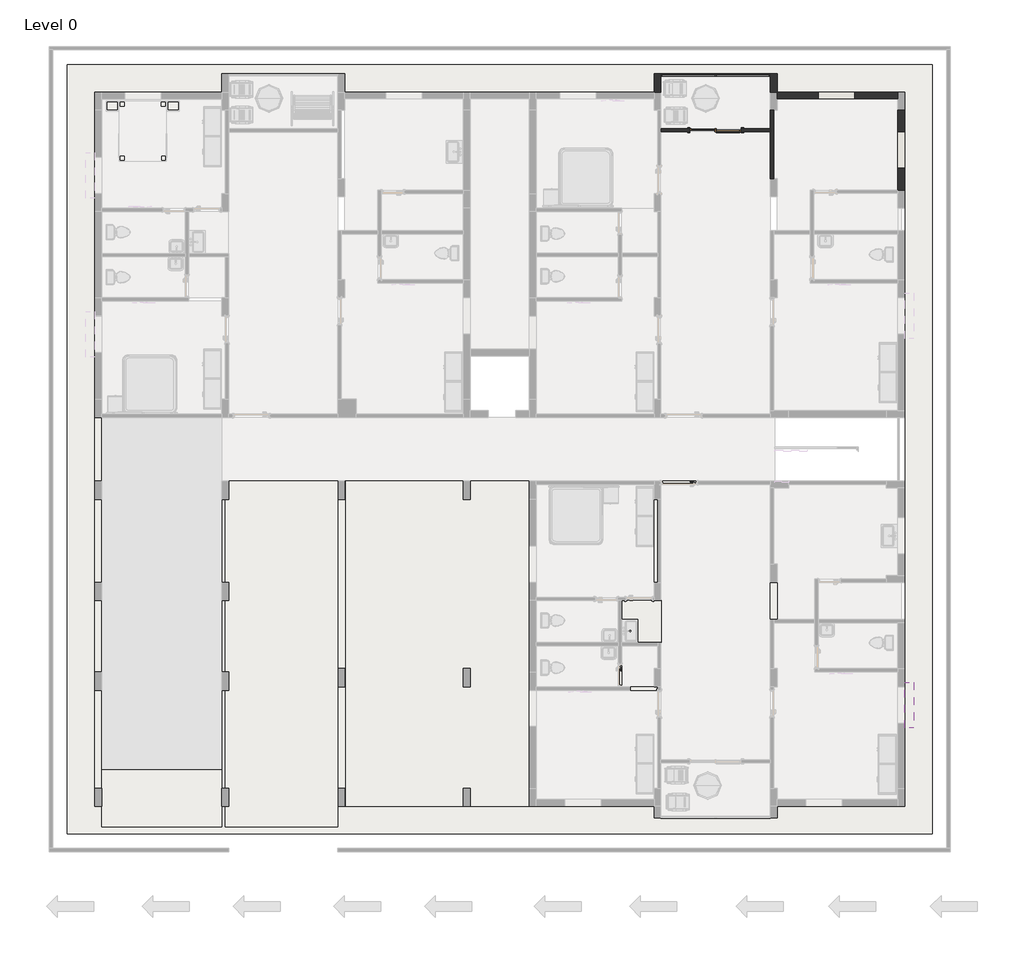
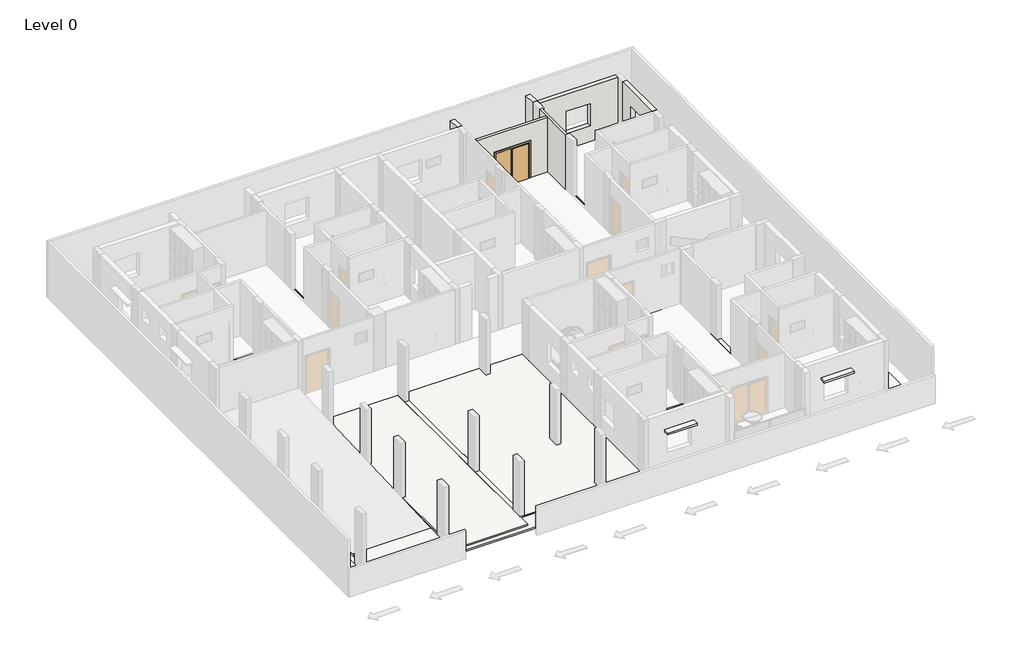
# One storey, part 3 of 6: 9 slabs, 7 walls, 5 members, 2 plates, 1 door.
"""IFC4 building model written with IfcOpenShell, lengths in millimetres."""

from ifc_helpers import new_model, si_unit, frame, origin, origin_with_axes, place, context, project, spatial, polyline, outline, extrude, faceted_brep, transform, mapped, element, save
from components import door_c5e969d5, rectangular_mullion_30mm_square_b78902bc, rectangular_mullion_30mm_square_5f4e9219, rectangular_mullion_30mm_square_f98953c9, rectangular_mullion_30mm_square_8997babb, system_panel_glazed_aa91312f, system_panel_glazed_e8634194

model = new_model("IFC4")

# Units and contexts
model_context = context("Model", 3, world=origin())
ifc_project = project(units=[si_unit("LENGTHUNIT", "METRE", prefix="MILLI")], contexts=[model_context])

# Site, building, storey
site = spatial("IfcSite", under=ifc_project)
building = spatial("IfcBuilding", under=site)
storey = spatial("IfcBuildingStorey", under=building, Name="Level 0", Elevation=0.0)

# Door
placement = place(None, origin())
door_shape = door_c5e969d5(model_context)
element("IfcDoor", 1, ObjectType="Door-Double-Sliding : 5'8\"", at=placement, inside=storey, context=model_context, shape_type="MappedRepresentation", body=[
    mapped(door_shape, transform((7286.1098461, 9214.7982139, 0.0), x_axis=(-1.0, 0.0, 0.0), y_axis=(0.0, -1.0, 0.0), z_axis=(0.0, 0.0, 1.0))),
])

# Members
rectangular_mullion_30mm_square_shape = rectangular_mullion_30mm_square_b78902bc(model_context)
element("IfcMember", 2, ObjectType="Rectangular Mullion : 30mm_Square", at=placement, inside=storey, context=model_context, shape_type="MappedRepresentation", body=[
    mapped(rectangular_mullion_30mm_square_shape, transform((7272.3098464, 10913.4232139, 1182.1950157), x_axis=(0.0, 0.0, 1.0), y_axis=(0.0, -1.0, 0.0), z_axis=(1.0, 0.0, 0.0))),
])
rectangular_mullion_30mm_square_2_shape = rectangular_mullion_30mm_square_5f4e9219(model_context)
element("IfcMember", 3, ObjectType="Rectangular Mullion : 30mm_Square", at=placement, inside=storey, context=model_context, shape_type="MappedRepresentation", body=[
    mapped(rectangular_mullion_30mm_square_2_shape, transform((9084.9098461, 10913.4232139, 1182.1950157), x_axis=(0.0, 0.0, 1.0), y_axis=(0.0, -1.0, 0.0), z_axis=(1.0, 0.0, 0.0))),
])
rectangular_mullion_30mm_square_3_shape = rectangular_mullion_30mm_square_f98953c9(model_context)
element("IfcMember", 4, ObjectType="Rectangular Mullion : 30mm_Square", at=placement, inside=storey, context=model_context, shape_type="MappedRepresentation", body=[
    mapped(rectangular_mullion_30mm_square_3_shape, transform((9114.9098461, 10913.4232139, 115.3950157), x_axis=(1.0, 0.0, 0.0), y_axis=(0.0, -1.0, 0.0), z_axis=(0.0, 0.0, -1.0))),
])
rectangular_mullion_30mm_square_4_shape = rectangular_mullion_30mm_square_8997babb(model_context)
element("IfcMember", 5, ObjectType="Rectangular Mullion : 30mm_Square", at=placement, inside=storey, context=model_context, shape_type="MappedRepresentation", body=[
    mapped(rectangular_mullion_30mm_square_4_shape, transform((7287.3098464, 10913.4232139, 115.3950157), x_axis=(1.0, 0.0, 0.0), y_axis=(0.0, -1.0, 0.0), z_axis=(0.0, 0.0, -1.0))),
])
element("IfcMember", 6, ObjectType="Rectangular Mullion : 30mm_Square", at=placement, inside=storey, context=model_context, shape_type="MappedRepresentation", body=[
    mapped(rectangular_mullion_30mm_square_3_shape, transform((5457.3098461, 10913.4232139, 1182.1950157), x_axis=(-1.0, 0.0, 0.0), y_axis=(0.0, -1.0, 0.0), z_axis=(0.0, 0.0, 1.0))),
])

# Plates
system_panel_glazed_shape = system_panel_glazed_aa91312f(model_context)
element("IfcPlate", 7, ObjectType="System Panel : Glazed", at=placement, inside=storey, context=model_context, shape_type="MappedRepresentation", body=[
    mapped(system_panel_glazed_shape, transform((8201.1098463, 10913.4232139, 115.3950157), x_axis=(1.0, 0.0, 0.0), y_axis=(0.0, 1.0, 0.0), z_axis=(0.0, 0.0, 1.0))),
])
system_panel_glazed_2_shape = system_panel_glazed_e8634194(model_context)
element("IfcPlate", 8, ObjectType="System Panel : Glazed", at=placement, inside=storey, context=model_context, shape_type="MappedRepresentation", body=[
    mapped(system_panel_glazed_2_shape, transform((6372.3098463, 10913.4232139, 115.3950157), x_axis=(1.0, 0.0, 0.0), y_axis=(0.0, 1.0, 0.0), z_axis=(0.0, 0.0, 1.0))),
])

# Slabs
element("IfcSlab", 9, at=placement, inside=storey, context=model_context, shape_type="Brep", body=[
    faceted_brep([(-5344.0401539, 9029.5022446, -50.8), (-5344.0401539, -406.5977554, -50.8), (-9001.6401539, -406.5977554, -50.8), (-9001.6401539, 4965.5022446, -50.8), (-9001.6401539, 6361.3562752, -50.8), (-9001.6401539, 9029.5022446, -50.8), (-5344.0401539, 9029.5022446, 0.0), (-9001.6401539, 9029.5022446, 0.0), (-9001.6401539, 6361.3562752, 0.0), (-9001.6401539, 4965.5022446, 0.0), (-9001.6401539, -406.5977554, 0.0), (-5344.0401539, -406.5977554, 0.0)], [[[0, 1, 2, 3, 4, 5]], [[6, 7, 8, 9, 10, 11]], [[1, 0, 6, 11]], [[2, 1, 11, 10]], [[5, 4, 3, 2, 10, 9, 8, 7]], [[0, 5, 7, 6]]]),
    faceted_brep([(-10450.1697227, 4851.2022446, -50.8), (-10450.1697227, 3479.6022446, -50.8), (-13249.7901539, 3479.6022446, -50.8), (-13249.7901539, 4851.2022446, -50.8), (-10450.1697227, 4851.2022446, 0.0), (-13249.7901539, 4851.2022446, 0.0), (-13249.7901539, 3479.6022446, 0.0), (-10450.1697227, 3479.6022446, 0.0)], [[[0, 1, 2, 3]], [[4, 5, 6, 7]], [[1, 0, 4, 7]], [[2, 1, 7, 6]], [[3, 2, 6, 5]], [[0, 3, 5, 4]]]),
    faceted_brep([(-10449.4401539, 6362.5022446, -50.8), (-10449.4401539, 4965.5022446, -50.8), (-13249.7901539, 4965.5022446, -50.8), (-13249.7901539, 6362.5022446, -50.8), (-10449.4401539, 6362.5022446, 0.0), (-13249.7901539, 6362.5022446, 0.0), (-13249.7901539, 4965.5022446, 0.0), (-10449.4401539, 4965.5022446, 0.0)], [[[0, 1, 2, 3]], [[4, 5, 6, 7]], [[1, 0, 4, 7]], [[2, 1, 7, 6]], [[3, 2, 6, 5]], [[0, 3, 5, 4]]]),
    faceted_brep([(-9230.2401539, 3365.3022446, -50.8), (-9230.2401539, 2871.1482139, -50.8), (-9115.9401539, 2871.1482139, -50.8), (-9115.9401539, 89.8788513, -50.8), (-9230.2401539, 89.8788513, -50.8), (-9230.2401539, -406.5977554, -50.8), (-13249.7901539, -406.5977554, -50.8), (-13249.7901539, 3365.3022446, -50.8), (-9230.2401539, 3365.3022446, 0.0), (-13249.7901539, 3365.3022446, 0.0), (-13249.7901539, -406.5977554, 0.0), (-9230.2401539, -406.5977554, 0.0), (-9230.2401539, 89.8788513, 0.0), (-9115.9401539, 89.8788513, 0.0), (-9115.9401539, 2871.1482139, 0.0), (-9230.2401539, 2871.1482139, 0.0)], [[[0, 1, 2, 3, 4, 5, 6, 7]], [[8, 9, 10, 11, 12, 13, 14, 15]], [[1, 0, 8, 15]], [[2, 1, 15, 14]], [[3, 2, 14, 13]], [[4, 3, 13, 12]], [[5, 4, 12, 11]], [[6, 5, 11, 10]], [[7, 6, 10, 9]], [[0, 7, 9, 8]]]),
    faceted_brep([(-9115.77783, 4851.2022446, -50.8), (-9115.77783, 3480.7482139, -50.8), (-10335.1401539, 3480.7482139, -50.8), (-10335.1401539, 4851.2022446, -50.8), (-9115.77783, 4851.2022446, 0.0), (-10335.1401539, 4851.2022446, 0.0), (-10335.1401539, 3480.7482139, 0.0), (-9115.77783, 3480.7482139, 0.0)], [[[0, 1, 2, 3]], [[4, 5, 6, 7]], [[1, 0, 4, 7]], [[2, 1, 7, 6]], [[3, 2, 6, 5]], [[0, 3, 5, 4]]]),
    faceted_brep([(-1153.0401539, 6972.4998276, -50.8), (-1153.0401539, 5727.5022446, -50.8), (-3895.589965, 5727.5022446, -50.8), (-3895.589965, 6972.4998276, -50.8), (-1153.0401539, 6972.4998276, 0.0), (-3895.589965, 6972.4998276, 0.0), (-3895.589965, 5727.5022446, 0.0), (-1153.0401539, 5727.5022446, 0.0)], [[[0, 1, 2, 3]], [[4, 5, 6, 7]], [[1, 0, 4, 7]], [[2, 1, 7, 6]], [[3, 2, 6, 5]], [[0, 3, 5, 4]]]),
    faceted_brep([(-1153.0702694, 10134.4022446, -50.8), (-1153.0702694, 7085.367621, -50.8), (-4009.8302587, 7086.8595027, -50.8), (-4010.5401539, 5727.5022446, -50.8), (-5115.4534022, 5727.5022446, -50.8), (-5115.4534022, 10134.4022446, -50.8), (-1153.0702694, 10134.4022446, 0.0), (-5115.4534022, 10134.4022446, 0.0), (-5115.4534022, 5727.5022446, 0.0), (-4010.5401539, 5727.5022446, 0.0), (-4009.8302587, 7086.8595027, 0.0), (-1153.0702694, 7085.367621, 0.0)], [[[0, 1, 2, 3, 4, 5]], [[6, 7, 8, 9, 10, 11]], [[1, 0, 6, 11]], [[2, 1, 11, 10]], [[3, 2, 10, 9]], [[4, 3, 9, 8]], [[5, 4, 8, 7]], [[0, 5, 7, 6]]]),
    faceted_brep([(-1153.0401539, 5613.2022446, -50.8), (-1153.0401539, 4089.2022446, -50.8), (-3896.2401539, 4089.2022446, -50.8), (-3896.2401539, 5613.2022446, -50.8), (-1153.0401539, 5613.2022446, 0.0), (-3896.2401539, 5613.2022446, 0.0), (-3896.2401539, 4089.2022446, 0.0), (-1153.0401539, 4089.2022446, 0.0)], [[[0, 1, 2, 3]], [[4, 5, 6, 7]], [[1, 0, 4, 7]], [[2, 1, 7, 6]], [[3, 2, 6, 5]], [[0, 3, 5, 4]]]),
    faceted_brep([(-5229.7401539, 5613.2022446, -50.8), (-4010.5998446, 5613.2022446, -50.8), (-4011.4554117, 3974.9022446, -50.8), (-1153.0401539, 3974.9022446, -50.8), (-1153.0401539, -406.5977554, -50.8), (-5229.7401539, -406.5977554, -50.8), (-5229.7401539, 5613.2022446, 0.0), (-5229.7401539, -406.5977554, 0.0), (-1153.0401539, -406.5977554, 0.0), (-1153.0401539, 3974.9022446, 0.0), (-4011.4554117, 3974.9022446, 0.0), (-4010.5998446, 5613.2022446, 0.0)], [[[0, 1, 2, 3, 4, 5]], [[6, 7, 8, 9, 10, 11]], [[1, 0, 6, 11]], [[2, 1, 11, 10]], [[3, 2, 10, 9]], [[4, 3, 9, 8]], [[5, 4, 8, 7]], [[0, 5, 7, 6]]]),
    faceted_brep([(1056.7598461, 10134.4022446, -50.8), (1056.7598461, 1766.2482139, -50.8), (-924.4401539, 1766.2482139, -50.8), (-924.4401539, 10134.4022446, -50.8), (1056.7598461, 10134.4022446, 0.0), (-924.4401539, 10134.4022446, 0.0), (-924.4401539, 1766.2482139, 0.0), (1056.7598461, 1766.2482139, 0.0)], [[[0, 1, 2, 3]], [[4, 5, 6, 7]], [[1, 0, 4, 7]], [[2, 1, 7, 6]], [[3, 2, 6, 5]], [[0, 3, 5, 4]]]),
    faceted_brep([(4028.5598461, 4852.3482139, -50.8), (4028.5598461, 3480.7482139, -50.8), (1285.3598461, 3480.7482139, -50.8), (1285.3598461, 4852.3482139, -50.8), (4028.5598461, 4852.3482139, 0.0), (1285.3598461, 4852.3482139, 0.0), (1285.3598461, 3480.7482139, 0.0), (4028.5598461, 3480.7482139, 0.0)], [[[0, 1, 2, 3]], [[4, 5, 6, 7]], [[1, 0, 4, 7]], [[2, 1, 7, 6]], [[3, 2, 6, 5]], [[0, 3, 5, 4]]]),
    faceted_brep([(1285.3598461, 4966.6482139, -50.8), (1285.3598461, 6362.5022446, -50.8), (4028.5598461, 6362.5022446, -50.8), (4028.5598461, 4966.6482139, -50.8), (1285.3598461, 4966.6482139, 0.0), (4028.5598461, 4966.6482139, 0.0), (4028.5598461, 6362.5022446, 0.0), (1285.3598461, 6362.5022446, 0.0)], [[[0, 1, 2, 3]], [[4, 5, 6, 7]], [[1, 0, 4, 7]], [[2, 1, 7, 6]], [[3, 2, 6, 5]], [[0, 3, 5, 4]]]),
    faceted_brep([(5228.7098461, 10134.4022446, -50.8), (5228.7098461, 9754.5482139, -50.8), (5343.0098461, 9754.5482139, -50.8), (5343.0098461, 6972.1022446, -50.8), (5228.7098461, 6972.1022446, -50.8), (5228.7098461, 6362.5022446, -50.8), (5343.0098461, 6362.5022446, -50.8), (5343.0098461, 4966.6482139, -50.8), (4142.8598461, 4966.6482139, -50.8), (4142.8598461, 6477.9482139, -50.8), (1285.3598461, 6477.9482139, -50.8), (1285.3598461, 10134.4022446, -50.8), (5228.7098461, 10134.4022446, 0.0), (1285.3598461, 10134.4022446, 0.0), (1285.3598461, 6477.9482139, 0.0), (4142.8598461, 6477.9482139, 0.0), (4142.8598461, 4966.6482139, 0.0), (5343.0098461, 4966.6482139, 0.0), (5343.0098461, 6362.5022446, 0.0), (5228.7098461, 6362.5022446, 0.0), (5228.7098461, 6972.1022446, 0.0), (5343.0098461, 6972.1022446, 0.0), (5343.0098461, 9754.5482139, 0.0), (5228.7098461, 9754.5482139, 0.0)], [[[0, 1, 2, 3, 4, 5, 6, 7, 8, 9, 10, 11]], [[12, 13, 14, 15, 16, 17, 18, 19, 20, 21, 22, 23]], [[1, 0, 12, 23]], [[2, 1, 23, 22]], [[3, 2, 22, 21]], [[4, 3, 21, 20]], [[5, 4, 20, 19]], [[6, 5, 19, 18]], [[7, 6, 18, 17]], [[8, 7, 17, 16]], [[9, 8, 16, 15]], [[10, 9, 15, 14]], [[11, 10, 14, 13]], [[0, 11, 13, 12]]]),
    faceted_brep([(4142.8598461, 3366.4482139, -50.8), (4142.8598461, 4852.3482139, -50.8), (5343.0098461, 4852.3482139, -50.8), (5343.0098461, 3481.8941832, -50.8), (5228.7098461, 3481.8941832, -50.8), (5228.7098461, 2872.2941832, -50.8), (5343.0098461, 2872.2941832, -50.8), (5343.0098461, 89.9385005, -50.8), (5228.7098461, 89.9385005, -50.8), (5228.7098461, -405.4517861, -50.8), (1285.3598461, -405.4517861, -50.8), (1285.3598461, 3366.4482139, -50.8), (4142.8598461, 3366.4482139, 0.0), (1285.3598461, 3366.4482139, 0.0), (1285.3598461, -405.4517861, 0.0), (5228.7098461, -405.4517861, 0.0), (5228.7098461, 89.9385005, 0.0), (5343.0098461, 89.9385005, 0.0), (5343.0098461, 2872.2941832, 0.0), (5228.7098461, 2872.2941832, 0.0), (5228.7098461, 3481.8941832, 0.0), (5343.0098461, 3481.8941832, 0.0), (5343.0098461, 4852.3482139, 0.0), (4142.8598461, 4852.3482139, 0.0)], [[[0, 1, 2, 3, 4, 5, 6, 7, 8, 9, 10, 11]], [[12, 13, 14, 15, 16, 17, 18, 19, 20, 21, 22, 23]], [[1, 0, 12, 23]], [[2, 1, 23, 22]], [[3, 2, 22, 21]], [[4, 3, 21, 20]], [[5, 4, 20, 19]], [[6, 5, 19, 18]], [[7, 6, 18, 17]], [[8, 7, 17, 16]], [[9, 8, 16, 15]], [[10, 9, 15, 14]], [[11, 10, 14, 13]], [[0, 11, 13, 12]]]),
    faceted_brep([(9114.9098461, 10898.4232139, -50.8), (9114.9098461, 9144.9482139, -50.8), (5457.3098461, 9144.9482139, -50.8), (5457.3098461, 10898.4232139, -50.8), (9114.9098461, 10898.4232139, 0.0), (5457.3098461, 10898.4232139, 0.0), (5457.3098461, 9144.9482139, 0.0), (9114.9098461, 9144.9482139, 0.0)], [[[0, 1, 2, 3]], [[4, 5, 6, 7]], [[1, 0, 4, 7]], [[2, 1, 7, 6]], [[3, 2, 6, 5]], [[0, 3, 5, 4]]]),
    faceted_brep([(9114.9098461, 9030.6482139, -50.8), (9114.9098461, -405.4517861, -50.8), (5457.3098461, -405.4517861, -50.8), (5457.3098461, 9030.6482139, -50.8), (9114.9098461, 9030.6482139, 0.0), (5457.3098461, 9030.6482139, 0.0), (5457.3098461, -405.4517861, 0.0), (9114.9098461, -405.4517861, 0.0)], [[[0, 1, 2, 3]], [[4, 5, 6, 7]], [[1, 0, 4, 7]], [[2, 1, 7, 6]], [[3, 2, 6, 5]], [[0, 3, 5, 4]]]),
    faceted_brep([(13382.1098461, 10135.5482139, -50.8), (13382.1098461, 7087.5482139, -50.8), (10448.4098461, 7087.5482139, -50.8), (10448.4098461, 5728.6482139, -50.8), (9346.6684396, 5728.6482139, -50.8), (9346.6684396, 7468.5482139, -50.8), (9229.2098461, 7468.5482139, -50.8), (9229.2098461, 9754.5482139, -50.8), (9343.5098461, 9754.5482139, -50.8), (9343.5098461, 10135.5482139, -50.8), (13382.1098461, 10135.5482139, 0.0), (9343.5098461, 10135.5482139, 0.0), (9343.5098461, 9754.5482139, 0.0), (9229.2098461, 9754.5482139, 0.0), (9229.2098461, 7468.5482139, 0.0), (9346.6684396, 7468.5482139, 0.0), (9346.6684396, 5728.6482139, 0.0), (10448.4098461, 5728.6482139, 0.0), (10448.4098461, 7087.5482139, 0.0), (13382.1098461, 7087.5482139, 0.0)], [[[0, 1, 2, 3, 4, 5, 6, 7, 8, 9]], [[10, 11, 12, 13, 14, 15, 16, 17, 18, 19]], [[1, 0, 10, 19]], [[2, 1, 19, 18]], [[3, 2, 18, 17]], [[4, 3, 17, 16]], [[5, 4, 16, 15]], [[6, 5, 15, 14]], [[7, 6, 14, 13]], [[8, 7, 13, 12]], [[9, 8, 12, 11]], [[0, 9, 11, 10]]]),
    faceted_brep([(10448.4098461, 5614.3482139, -50.8), (10448.4098461, 3976.0482139, -50.8), (13382.1098461, 3976.0482139, -50.8), (13382.1098461, 3480.7482139, -50.8), (13382.1098461, -291.1517861, -50.8), (9229.2098461, -291.1517861, -50.8), (9229.2098461, 3480.7482139, -50.8), (9343.5098461, 3480.7482139, -50.8), (9343.5098461, 4090.3482139, -50.8), (9229.2098461, 4090.3482139, -50.8), (9229.2098461, 5614.3482139, -50.8), (10448.4098461, 5614.3482139, 0.0), (9229.2098461, 5614.3482139, 0.0), (9229.2098461, 4090.3482139, 0.0), (9343.5098461, 4090.3482139, 0.0), (9343.5098461, 3480.7482139, 0.0), (9229.2098461, 3480.7482139, 0.0), (9229.2098461, -291.1517861, 0.0), (13382.1098461, -291.1517861, 0.0), (13382.1098461, 3480.7482139, 0.0), (13382.1098461, 3976.0482139, 0.0), (10448.4098461, 3976.0482139, 0.0)], [[[0, 1, 2, 3, 4, 5, 6, 7, 8, 9, 10]], [[11, 12, 13, 14, 15, 16, 17, 18, 19, 20, 21]], [[1, 0, 11, 21]], [[2, 1, 21, 20]], [[3, 2, 20, 19]], [[4, 3, 19, 18]], [[5, 4, 18, 17]], [[6, 5, 17, 16]], [[7, 6, 16, 15]], [[8, 7, 15, 14]], [[9, 8, 14, 13]], [[10, 9, 13, 12]], [[0, 10, 12, 11]]]),
    faceted_brep([(13382.1098461, 5614.3482139, -50.8), (13382.1098461, 4090.3482139, -50.8), (10562.7098461, 4090.3482139, -50.8), (10562.7098461, 5614.3482139, -50.8), (13382.1098461, 5614.3482139, 0.0), (10562.7098461, 5614.3482139, 0.0), (10562.7098461, 4090.3482139, 0.0), (13382.1098461, 4090.3482139, 0.0)], [[[0, 1, 2, 3]], [[4, 5, 6, 7]], [[1, 0, 4, 7]], [[2, 1, 7, 6]], [[3, 2, 6, 5]], [[0, 3, 5, 4]]]),
    faceted_brep([(-9230.2401539, 10133.2562752, -50.8), (-9230.2401539, 9752.2562752, -50.8), (-9115.9401539, 9752.2562752, -50.8), (-9115.9401539, 6972.1022446, -50.8), (-9230.2401539, 6972.1022446, -50.8), (-9230.2401539, 6476.8022446, -50.8), (-13249.7901539, 6476.8022446, -50.8), (-13249.7901539, 10133.2562752, -50.8), (-9230.2401539, 10133.2562752, 0.0), (-13249.7901539, 10133.2562752, 0.0), (-13249.7901539, 6476.8022446, 0.0), (-9230.2401539, 6476.8022446, 0.0), (-9230.2401539, 6972.1022446, 0.0), (-9115.9401539, 6972.1022446, 0.0), (-9115.9401539, 9752.2562752, 0.0), (-9230.2401539, 9752.2562752, 0.0)], [[[0, 1, 2, 3, 4, 5, 6, 7]], [[8, 9, 10, 11, 12, 13, 14, 15]], [[5, 4, 12, 11]], [[6, 5, 11, 10]], [[7, 6, 10, 9]], [[0, 7, 9, 8]], [[1, 0, 8, 15]], [[2, 1, 15, 14]], [[3, 2, 14, 13]], [[4, 3, 13, 12]]]),
    faceted_brep([(1056.7598461, -2653.3517861, -50.8), (1056.7598461, -13537.2517861, -50.8), (-9001.6401539, -13537.2517861, -50.8), (-9001.6401539, -12927.6517861, -50.8), (-9001.6401539, -9651.0517861, -50.8), (-9001.6401539, -9041.4517861, -50.8), (-9001.6401539, -6653.8517861, -50.8), (-9001.6401539, -6044.2517861, -50.8), (-9001.6401539, -3262.9517861, -50.8), (-9001.6401539, -2653.3517861, -50.8), (1056.7598461, -2653.3517861, 0.0), (-9001.6401539, -2653.3517861, 0.0), (-9001.6401539, -3262.9517861, 0.0), (-9001.6401539, -6044.2517861, 0.0), (-9001.6401539, -6653.8517861, 0.0), (-9001.6401539, -9041.4517861, 0.0), (-9001.6401539, -9651.0517861, 0.0), (-9001.6401539, -12927.6517861, 0.0), (-9001.6401539, -13537.2517861, 0.0), (1056.7598461, -13537.2517861, 0.0)], [[[0, 1, 2, 3, 4, 5, 6, 7, 8, 9]], [[10, 11, 12, 13, 14, 15, 16, 17, 18, 19]], [[1, 0, 10, 19]], [[2, 1, 19, 18]], [[9, 8, 7, 6, 5, 4, 3, 2, 18, 17, 16, 15, 14, 13, 12, 11]], [[0, 9, 11, 10]]]),
    faceted_brep([(5228.7098461, -2767.0150775, -50.8), (5228.7098461, -6539.5517861, -50.8), (1285.3598461, -6539.5517861, -50.8), (1285.3598461, -2767.0150775, -50.8), (5228.7098461, -2767.0150775, 0.0), (1285.3598461, -2767.0150775, 0.0), (1285.3598461, -6539.5517861, 0.0), (5228.7098461, -6539.5517861, 0.0)], [[[0, 1, 2, 3]], [[4, 5, 6, 7]], [[1, 0, 4, 7]], [[2, 1, 7, 6]], [[3, 2, 6, 5]], [[0, 3, 5, 4]]]),
    faceted_brep([(9114.9098461, -2767.6517861, -50.8), (9114.9098461, -11975.1517861, -50.8), (5462.3098461, -11975.1517861, -50.8), (5462.3098461, -10565.4518735, -50.8), (5462.3098461, -9651.0517861, -50.8), (5462.3098461, -8050.8607795, -50.8), (5462.3098461, -6653.8517861, -50.8), (5462.3098461, -2767.6517861, -50.8), (9114.9098461, -2767.6517861, 0.0), (5462.3098461, -2767.6517861, 0.0), (5462.3098461, -6653.8517861, 0.0), (5462.3098461, -8050.8607795, 0.0), (5462.3098461, -9651.0517861, 0.0), (5462.3098461, -10565.4518735, 0.0), (5462.3098461, -11975.1517861, 0.0), (9114.9098461, -11975.1517861, 0.0)], [[[0, 1, 2, 3, 4, 5, 6, 7]], [[8, 9, 10, 11, 12, 13, 14, 15]], [[1, 0, 8, 15]], [[2, 1, 15, 14]], [[7, 6, 5, 4, 3, 2, 14, 13, 12, 11, 10, 9]], [[0, 7, 9, 8]]]),
    faceted_brep([(9343.5098461, -7288.8517861, -50.8), (9343.5098461, -6044.2517861, -50.8), (9343.5098461, -5434.6517861, -50.8), (9229.2098461, -5434.6517861, -50.8), (9229.2098461, -2881.9517861, -50.8), (9725.7585903, -2881.9517861, -50.8), (9725.7585903, -2767.6517861, -50.8), (13001.1098461, -2767.6517861, -50.8), (13001.1098461, -2881.9517861, -50.8), (13382.1098461, -2881.9517861, -50.8), (13382.1098461, -5815.6517861, -50.8), (13001.1098461, -5815.6517861, -50.8), (13001.1098461, -5929.9517861, -50.8), (10600.8098461, -5929.9517861, -50.8), (10600.8098461, -7288.8517861, -50.8), (9343.5098461, -7288.8517861, 0.0), (10600.8098461, -7288.8517861, 0.0), (10600.8098461, -5929.9517861, 0.0), (13001.1098461, -5929.9517861, 0.0), (13001.1098461, -5815.6517861, 0.0), (13382.1098461, -5815.6517861, 0.0), (13382.1098461, -2881.9517861, 0.0), (13001.1098461, -2881.9517861, 0.0), (13001.1098461, -2767.6517861, 0.0), (9725.7585903, -2767.6517861, 0.0), (9725.7585903, -2881.9517861, 0.0), (9229.2098461, -2881.9517861, 0.0), (9229.2098461, -5434.6517861, 0.0), (9343.5098461, -5434.6517861, 0.0), (9343.5098461, -6044.2517861, 0.0)], [[[0, 1, 2, 3, 4, 5, 6, 7, 8, 9, 10, 11, 12, 13, 14]], [[15, 16, 17, 18, 19, 20, 21, 22, 23, 24, 25, 26, 27, 28, 29]], [[1, 0, 15, 29]], [[2, 1, 29, 28]], [[3, 2, 28, 27]], [[4, 3, 27, 26]], [[5, 4, 26, 25]], [[6, 5, 25, 24]], [[7, 6, 24, 23]], [[8, 7, 23, 22]], [[9, 8, 22, 21]], [[10, 9, 21, 20]], [[11, 10, 20, 19]], [[12, 11, 19, 18]], [[13, 12, 18, 17]], [[14, 13, 17, 16]], [[0, 14, 16, 15]]]),
    faceted_brep([(9114.9098461, -12089.4517861, -50.8), (9114.9098461, -13867.4517861, -50.8), (5457.3098461, -13867.4517861, -50.8), (5457.3098461, -12089.4517861, -50.8), (9114.9098461, -12089.4517861, 0.0), (5457.3098461, -12089.4517861, 0.0), (5457.3098461, -13867.4517861, 0.0), (9114.9098461, -13867.4517861, 0.0)], [[[0, 1, 2, 3]], [[4, 5, 6, 7]], [[1, 0, 4, 7]], [[2, 1, 7, 6]], [[3, 2, 6, 5]], [[0, 3, 5, 4]]]),
    faceted_brep([(13382.1098461, -7403.1517861, -50.8), (13382.1098461, -8927.1517861, -50.8), (10715.1098461, -8927.1517861, -50.8), (10715.1098461, -7403.1517861, -50.8), (13382.1098461, -7403.1517861, 0.0), (10715.1098461, -7403.1517861, 0.0), (10715.1098461, -8927.1517861, 0.0), (13382.1098461, -8927.1517861, 0.0)], [[[0, 1, 2, 3]], [[4, 5, 6, 7]], [[1, 0, 4, 7]], [[2, 1, 7, 6]], [[3, 2, 6, 5]], [[0, 3, 5, 4]]]),
    faceted_brep([(9343.5098461, -13308.6517861, -50.8), (9343.5098461, -12927.6517861, -50.8), (9229.2098461, -12927.6517861, -50.8), (9229.2098461, -9536.7517861, -50.8), (9343.5098461, -9536.7517861, -50.8), (9343.5098461, -8927.1517861, -50.8), (9229.2098461, -8927.1517861, -50.8), (9229.2098461, -7403.1517861, -50.8), (10600.8098461, -7403.1517861, -50.8), (10600.8098461, -9041.4517861, -50.8), (13382.1098461, -9041.4517861, -50.8), (13382.1098461, -13308.6517861, -50.8), (9343.5098461, -13308.6517861, 0.0), (13382.1098461, -13308.6517861, 0.0), (13382.1098461, -9041.4517861, 0.0), (10600.8098461, -9041.4517861, 0.0), (10600.8098461, -7403.1517861, 0.0), (9229.2098461, -7403.1517861, 0.0), (9229.2098461, -8927.1517861, 0.0), (9343.5098461, -8927.1517861, 0.0), (9343.5098461, -9536.7517861, 0.0), (9229.2098461, -9536.7517861, 0.0), (9229.2098461, -12927.6517861, 0.0), (9343.5098461, -12927.6517861, 0.0)], [[[0, 1, 2, 3, 4, 5, 6, 7, 8, 9, 10, 11]], [[12, 13, 14, 15, 16, 17, 18, 19, 20, 21, 22, 23]], [[1, 0, 12, 23]], [[2, 1, 23, 22]], [[3, 2, 22, 21]], [[4, 3, 21, 20]], [[5, 4, 20, 19]], [[6, 5, 19, 18]], [[7, 6, 18, 17]], [[8, 7, 17, 16]], [[9, 8, 16, 15]], [[10, 9, 15, 14]], [[11, 10, 14, 13]], [[0, 11, 13, 12]]]),
])
element("IfcSlab", 10, at=placement, inside=storey, context=model_context, shape_type="SweptSolid", body=[
    extrude(outline(polyline([(-9115.9401539, -520.8977554), (-9115.9401539, -2653.3517861), (-9230.2401539, -2653.3517861), (-9230.2401539, -3262.9517861), (-9001.6401539, -3262.9517861), (-9001.6401539, -6044.2517861), (-9230.2401539, -6044.2517861), (-9230.2401539, -6653.8517861), (-9001.6401539, -6653.8517861), (-9001.6401539, -9041.4517861), (-9230.2401539, -9041.4517861), (-9230.2401539, -9651.0517861), (-9001.6401539, -9651.0517861), (-9001.6401539, -12927.6517861), (-9230.2401539, -12927.6517861), (-9230.2401539, -13537.2517861), (-13249.7901539, -13537.2517861), (-13249.7901539, -12927.6517861), (-13478.3901539, -12927.6517861), (-13478.3901539, -9651.0211487), (-13249.7901539, -9651.0211487), (-13249.7901539, -9041.4517861), (-13478.3901539, -9041.4517861), (-13478.3901539, -6653.8517861), (-13249.7901539, -6653.8517861), (-13249.7901539, -6044.2517861), (-13478.3901539, -6044.2517861), (-13478.3901539, -3262.9517861), (-13249.7901539, -3262.9517861), (-13249.7901539, -2653.3517861), (-13478.3901539, -2653.3517861), (-13478.3901539, -520.8977554), (-9115.9401539, -520.8977554)])), frame((0.0, 0.0, -50.8), z_axis=(0.0, 0.0, 1.0), x_axis=(1.0, 0.0, 0.0)), (0.0, 0.0, 1.0), 50.8),
])
element("IfcSlab", 11, ObjectType="4\"", at=placement, inside=storey, context=model_context, shape_type="SweptSolid", body=[
    extrude(outline(polyline([(13610.7098461, -3721.2859152), (13915.5098465, -3721.2859152), (13915.5098465, -5245.2859152), (13610.7098461, -5245.2859152), (13610.7098461, -3721.2859152)])), frame((0.0, 0.0, 2108.2), z_axis=(0.0, 0.0, 1.0), x_axis=(1.0, 0.0, 0.0)), (0.0, 0.0, 1.0), 101.6),
    extrude(outline(polyline([(13915.5098465, -9384.9129305), (13915.5098465, -10908.9129305), (13610.7098461, -10908.9129305), (13610.7098461, -9384.9129305), (13915.5098465, -9384.9129305)])), frame((0.0, 0.0, 2108.2), z_axis=(0.0, 0.0, 1.0), x_axis=(1.0, 0.0, 0.0)), (0.0, 0.0, 1.0), 101.6),
    extrude(outline(polyline([(10141.8125904, -13537.2517861), (11665.8125904, -13537.2517861), (11665.8125904, -13842.0517862), (10141.8125904, -13842.0517862), (10141.8125904, -13537.2517861)])), frame((0.0, 0.0, 2108.2), z_axis=(0.0, 0.0, 1.0), x_axis=(1.0, 0.0, 0.0)), (0.0, 0.0, 1.0), 101.6),
    extrude(outline(polyline([(2083.6625904, -13537.2517861), (3607.6625904, -13537.2517861), (3607.6625904, -13842.0517862), (2083.6625904, -13842.0517862), (2083.6625904, -13537.2517861)])), frame((0.0, 0.0, 2108.2), z_axis=(0.0, 0.0, 1.0), x_axis=(1.0, 0.0, 0.0)), (0.0, 0.0, 1.0), 101.6),
])
element("IfcSlab", 12, ObjectType="4\"", at=placement, inside=storey, context=model_context, shape_type="SweptSolid", body=[
    extrude(outline(polyline([(-14392.189503, 11278.5482139), (14525.710497, 11278.5482139), (14525.710497, -14451.6517861), (-14392.189503, -14451.6517861), (-14392.189503, 11278.5482139)]), holes=[polyline([(13610.7098461, -13537.2517861), (13610.7098461, 10364.1482139), (9343.5098461, 10364.1482139), (9343.5098461, 10973.7482139), (5228.7098461, 10973.7482139), (5228.7098461, 10363.0022446), (-5115.4534022, 10363.0022446), (-5115.4534022, 10972.6022446), (-9229.64062, 10972.6022446), (-9229.64062, 10361.8562752), (-13478.3901539, 10361.8562752), (-13478.3901539, -480.5643541), (-13478.3901539, -13537.2517861), (-3608.2937127, -13537.2517861), (5229.30938, -13537.2517861), (5229.30938, -13918.2517861), (5457.90938, -13918.2517861), (5457.90938, -13933.2517861), (9114.9098461, -13933.2517861), (9114.9098461, -13918.2517861), (9343.5098461, -13918.2517861), (9343.5098461, -13537.2517861), (13610.7098461, -13537.2517861)])]), frame((0.0, 0.0, -101.6), z_axis=(0.0, 0.0, 1.0), x_axis=(1.0, 0.0, 0.0)), (0.0, 0.0, 1.0), 101.6),
])
element("IfcSlab", 13, ObjectType="Tile", at=placement, inside=storey, context=model_context, shape_type="SweptSolid", body=[
    extrude(outline(polyline([(-9233.4151539, -2653.3517861), (-9233.4151539, -14223.0543293), (-13249.7901539, -14223.0543293), (-13249.7901539, -2653.3517861), (-9233.4151539, -2653.3517861)])), origin_with_axes(), (0.0, 0.0, 1.0), 76.2),
    extrude(outline(polyline([(-9115.9534021, -2653.3517862), (-5343.44062, -2653.3517862), (-5343.44062, -14223.0543293), (-9115.9534021, -14223.0543293), (-9115.9534021, -2653.3517862)])), origin_with_axes(), (0.0, 0.0, 1.0), 76.2),
    extrude(outline(polyline([(1285.3598461, -2653.3517861), (1285.3598461, -13537.2517861), (-5085.1392999, -13537.2517861), (-5085.1392999, -2653.3517861), (1285.3598461, -2653.3517861)])), origin_with_axes(), (0.0, 0.0, 1.0), 76.2),
])
element("IfcSlab", 14, ObjectType="Tile", at=placement, inside=storey, context=model_context, shape_type="SweptSolid", body=[
    extrude(outline(polyline([(5462.3098461, -6653.8517861), (5462.3098461, -8050.8607795), (4142.8598461, -8050.8607795), (4142.8598461, -6653.8517861), (5462.3098461, -6653.8517861)])), origin_with_axes(), (0.0, 0.0, 1.0), 76.2),
])
element("IfcSlab", 15, ObjectType="Tile", at=placement, inside=storey, context=model_context, shape_type="SweptSolid", body=[
    extrude(outline(polyline([(-5085.1392999, -2653.3517862), (-5085.1392999, -13537.2517861), (-5343.44062, -13537.2517861), (-5343.44062, -2653.3517862), (-5085.1392999, -2653.3517862)])), origin_with_axes(), (0.0, 0.0, 1.0), 76.2),
])
element("IfcSlab", 16, ObjectType="Tile", at=placement, inside=storey, context=model_context, shape_type="SweptSolid", body=[
    extrude(outline(polyline([(9343.5098461, -5434.6517861), (9343.5098461, -7288.8517861), (9114.9098461, -7288.8517861), (9114.9098461, -5434.6517861), (9343.5098461, -5434.6517861)])), origin_with_axes(), (0.0, 0.0, 1.0), 76.2),
    extrude(outline(polyline([(5228.7098461, -3262.9517861), (5457.3098461, -3262.9517861), (5457.3098461, -6653.8517861), (5228.7098461, -6653.8517861), (5228.7098461, -3262.9517861)])), origin_with_axes(), (0.0, 0.0, 1.0), 76.2),
    extrude(outline(polyline([(9114.9098461, -2653.3517861), (9114.9098461, -2767.6517861), (5457.3098461, -2767.6517861), (5457.3098461, -2653.3517861), (9114.9098461, -2653.3517861)])), origin_with_axes(), (0.0, 0.0, 1.0), 76.2),
])
element("IfcSlab", 17, ObjectType="Tile", at=placement, inside=storey, context=model_context, shape_type="SweptSolid", body=[
    extrude(outline(polyline([(5343.0098461, -9536.7517861), (5343.0098461, -9651.0517861), (4428.2038363, -9651.0517861), (4428.2038363, -9536.7517861), (5343.0098461, -9536.7517861)])), origin_with_axes(), (0.0, 0.0, 1.0), 76.2),
    extrude(outline(polyline([(4142.8598461, -8774.7517861), (4142.8598461, -9536.7517862), (4028.5598461, -9536.7517862), (4028.5598461, -8774.7517861), (4142.8598461, -8774.7517861)])), origin_with_axes(), (0.0, 0.0, 1.0), 76.2),
])

# Walls
element("IfcWall", 18, ObjectType="2\"", at=placement, inside=storey, context=model_context, shape_type="SweptSolid", body=[
    extrude(outline(polyline([(9114.9098461, 10922.9482139), (5457.3098461, 10922.9482139), (5457.3098461, 10973.7482139), (9114.9098461, 10973.7482139), (9114.9098461, 10922.9482139)])), origin_with_axes(), (0.0, 0.0, 1.0), 115.3950157),
])
element("IfcWall", 19, ObjectType="9\"", at=placement, inside=storey, context=model_context, shape_type="SweptSolid", body=[
    extrude(outline(polyline([(0.0, 9343.5098461), (0.0, 13382.1098461), (3048.0, 13382.1098461), (3048.0, 9343.5098461), (0.0, 9343.5098461)]), holes=[polyline([(2133.6, 10715.1098462), (2133.6, 11934.3098462), (914.4, 11934.3098462), (914.4, 10715.1098462), (2133.6, 10715.1098462)])]), frame((0.0, 10135.5482139, 0.0), z_axis=(0.0, 1.0, 0.0), x_axis=(0.0, 0.0, 1.0)), (0.0, 0.0, 1.0), 228.6),
])
element("IfcWall", 20, ObjectType="9\"", at=placement, inside=storey, context=model_context, shape_type="SweptSolid", body=[
    extrude(outline(polyline([(7086.4022446, 0.0), (7086.4022446, 3048.0), (9754.5482139, 3048.0), (9754.5482139, 0.0), (7086.4022446, 0.0)]), holes=[polyline([(9030.0752292, 2133.6), (7810.8752292, 2133.6), (7810.8752292, 914.4), (9030.0752292, 914.4), (9030.0752292, 2133.6)])]), frame((13382.1098461, 0.0, 0.0), z_axis=(1.0, 0.0, 0.0), x_axis=(0.0, 1.0, 0.0)), (0.0, 0.0, 1.0), 228.6),
])
element("IfcWall", 21, ObjectType="9\"", at=placement, inside=storey, context=model_context, shape_type="SweptSolid", body=[
    extrude(outline(polyline([(5228.7098461, 10973.7482139), (5457.3098461, 10973.7482139), (5457.3098461, 10364.1482139), (5228.7098461, 10364.1482139), (5228.7098461, 10973.7482139)])), origin_with_axes(), (0.0, 0.0, 1.0), 3048.0),
])
element("IfcWall", 22, ObjectType="9\"", at=placement, inside=storey, context=model_context, shape_type="SweptSolid", body=[
    extrude(outline(polyline([(9343.5098461, 10973.7482139), (9343.5098461, 10364.1482139), (9114.9098461, 10364.1482139), (9114.9098461, 10973.7482139), (9343.5098461, 10973.7482139)])), origin_with_axes(), (0.0, 0.0, 1.0), 3048.0),
])
element("IfcWall", 23, ObjectType="Brick Wall 4.5\"", at=placement, inside=storey, context=model_context, shape_type="SweptSolid", body=[
    extrude(outline(polyline([(0.0, 5457.3098461), (0.0, 6422.5098461), (2032.0, 6422.5098461), (2032.0, 8149.7098461), (0.0, 8149.7098461), (0.0, 9114.9098461), (3048.0, 9114.9098461), (3048.0, 5457.3098461), (0.0, 5457.3098461)])), frame((0.0, 9030.6482139, 0.0), z_axis=(0.0, 1.0, 0.0), x_axis=(0.0, 0.0, 1.0)), (0.0, 0.0, 1.0), 114.3),
])
element("IfcWall", 24, ObjectType="Brick Wall 4.5\"", at=placement, inside=storey, context=model_context, shape_type="Brep", body=[
    faceted_brep([(9229.2098461, 7468.5482139, 0.0), (9229.2098461, 9753.4022446, 0.0), (9229.2098461, 9753.4022446, 3048.0), (9229.2098461, 7468.5482139, 3048.0), (9114.9098461, 7468.5482139, 0.0), (9114.9098461, 7468.5482139, 3048.0), (9114.9098461, 9030.6482139, 3048.0), (9114.9098461, 9144.9482139, 3048.0), (9114.9098461, 9753.4022446, 3048.0), (9114.9098461, 9753.4022446, 0.0), (9114.9098461, 9144.9482139, 0.0), (9114.9098461, 9030.6482139, 0.0)], [[[0, 1, 2, 3]], [[4, 5, 6, 7, 8, 9, 10, 11]], [[1, 0, 4, 11, 10, 9]], [[2, 1, 9, 8]], [[3, 2, 8, 7, 6, 5]], [[0, 3, 5, 4]]]),
])

save(model, "model.ifc")

# Revit data of these elements
# Type "Door-Double-Sliding : 5'8\""
#   Type Mark = "51"
#   Construction Type Id = "opn-d45"
#   Assembly Code = "C1020"
#   Analytic Construction = "Wood frame, double glass door "
#   Thickness = 0' - 2"
#   Thermal Resistance (R) = 0.31964 (m²·K)/W
#   Heat Transfer Coefficient (U) = 3.12872 W/(m²·K)
#   Height = 6' - 8"
#   Rail Width = 0' - 2"
#   Stiles = 0' - 2"
#   Trim Projection Ext = 0' - 1"
#   Trim Projection Int = 0' - 1"
#   Trim Width = 0' - 3"
#   Width = 5' - 8"
#   Define Thermal Properties by = 1
#   Glazing = Glass
#   Panel Material = Wood - Birch - Solid Stained Light Low Gloss
#   Trim Material = Paint - Sienna
#   Visual Light Transmittance = 0
#   Solar Heat Gain Coefficient = 0
#   Function = (empty or 0)
#   Wall Closure = (empty or 0)
# Type "Rectangular Mullion : 30mm_Square"
#   Keynote = "H11"
#   built-in parameter 1007304 = 0.0984252 (stored number, unit not read)
#   built-in parameter 1007301 = 0.0492126 (stored number, unit not read)
#   built-in parameter 1007300 = 0.0492126 (stored number, unit not read)
# Type "System Panel : Glazed"
#   Keynote = "H11"
#   Construction Type Id = "GSP4R"
#   Analytic Construction = "1/8 in Pilkington single glazing"
#   Visual Light Transmittance = 0.9
#   Solar Heat Gain Coefficient = 0.86
#   Heat Transfer Coefficient (U) = 6.7069 W/(m²·K)
#   Define Thermal Properties by = 1
# Type
#   Function = 0
#   Layers, outside or top first: 0' - 2" "Concrete" (function 1)
# Type "4\""
#   Function = 0
#   Layers, outside or top first: 0' - 4" "Concrete" (function 1)
# Type "Tile"
#   Function = 0
#   Layers, outside or top first: 0' - 2" "Sand" (function 1); 0' - 1" "Sand" (function 1)
# Type "2\""
#   Keynote = "F10"
#   Layers, outside or top first: 0' - 2" "Concrete" (function 1)
# Type "9\""
#   Keynote = "F10"
#   Layers, outside or top first: 0' - 9" "Concrete" (function 1)
# Type "Brick Wall 4.5\""
#   Keynote = "F10"
#   Layers, outside or top first: 0' - 4 1/2" "Brick, Engineering" (function 1)
# Element 1 (IfcDoor, "Door-Double-Sliding : 5'8\"")
#   Phase Created = New Construction
#   Materials on its faces: "Paint - Sienna", "Wood - Birch - Solid Stained Light Low Gloss", "Glass"
# Elements 2, 3, 4, 5, 6 (IfcMember, "Rectangular Mullion : 30mm_Square")
#   Phase Created = New Construction
#   Materials on its faces: "Aluminium"
# Elements 7, 8 (IfcPlate, "System Panel : Glazed")
#   Phase Created = New Construction
#   Materials on its faces: "Glass"
# Elements 9, 10 (IfcSlab)
#   Height Offset From Level = 0' - 0"
#   Phase Created = New Construction
#   Materials on its faces: "Concrete"
# Element 11 (IfcSlab, "4\"")
#   built-in parameter 1001955 = 1.5708 (stored number, unit not read)
#   Height Offset From Level = 7' - 3"
#   Phase Created = New Construction
#   Materials on its faces: "Concrete"
# Element 12 (IfcSlab, "4\"")
#   built-in parameter 1001955 = 1.5708 (stored number, unit not read)
#   Height Offset From Level = 0' - 0"
#   Phase Created = New Construction
#   Materials on its faces: "Concrete"
# Elements 13, 14, 15, 16, 17 (IfcSlab, "Tile")
#   Height Offset From Level = 0' - 3"
#   Phase Created = New Construction
#   Materials on its faces: "Sand"
# Element 18 (IfcWall, "2\"")
#   Top Offset = -9' - 7.45689"
#   Base Offset = 0' - 0"
#   wall height = 0' - 4.54311"
#   Phase Created = New Construction
#   Base Constraint = Level 0
#   Top Constraint = Level 1
#   Materials on its faces: "Concrete"
# Elements 19, 20, 21, 22 (IfcWall, "9\"")
#   Top Offset = 0' - 0"
#   Base Offset = 0' - 0"
#   wall height = 10' - 0"
#   Phase Created = New Construction
#   Base Constraint = Level 0
#   Top Constraint = Level 1
#   Materials on its faces: "Concrete"
# Elements 23, 24 (IfcWall, "Brick Wall 4.5\"")
#   Top Offset = 0' - 0"
#   Base Offset = 0' - 0"
#   wall height = 10' - 0"
#   Phase Created = New Construction
#   Base Constraint = Level 0
#   Top Constraint = Level 1
#   Materials on its faces: "Brick, Engineering"
# Materials
#   "Glass": class "Glass", colour RGB 0 128 192, transparency 0.9, Description = "Soda Lime Glass", Cost = 0
#   "Wood - Birch - Solid Stained Light Low Gloss": class "Wood", colour RGB 210 159 95, transparency 0, Cost = 0
#   "Paint - Sienna": colour RGB 118 70 51, transparency 0, Cost = 0
#   "Concrete": class "Concrete", colour RGB 120 120 120, transparency 0, Description = "Portland Cement Concrete", Cost = 0
#   "Sand": class "Generic", colour RGB 255 255 130, transparency 0, Description = "Sand", Cost = 0
#   "Brick, Engineering": class "Masonry", colour RGB 255 125 125, transparency 0, Description = "High fired, dense brick", Cost = 0
#   "Aluminium": class "Metal", colour RGB 247 247 247, transparency 0, Description = "Aluminium 6061", Cost = 0
